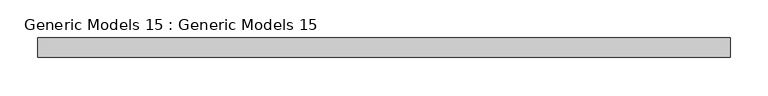
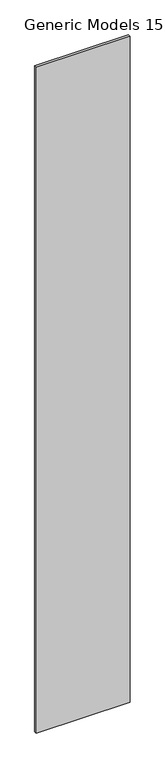
"""IFC4 building model written with IfcOpenShell, lengths in millimetres: proxy geometry, Generic Models 15 : Generic Models 15."""

from ifc_helpers import new_model, si_unit, frame, origin, place, context, project, spatial, polyline, outline, extrude, source, transform, mapped, element, save


def generic_models_15_generic_models_15_a6985b4b(model_context):
    return source(origin(), model_context, "Body", "SweptSolid", [
        extrude(outline(polyline([(-15207.3371373, -3405.661407), (-16121.7371373, -3405.661407), (-16121.7371373, -3380.261407), (-15207.3371373, -3380.261407), (-15207.3371373, -3405.661407)])), frame((0.0, 0.0, 304.8), z_axis=(0.0, 0.0, 1.0), x_axis=(1.0, 0.0, 0.0)), (0.0, 0.0, 1.0), 6858.0),
    ])


if __name__ == "__main__":
    model = new_model("IFC4")
    model_context = context("Model", 3, world=origin())
    ifc_project = project(units=[si_unit("LENGTHUNIT", "METRE", prefix="MILLI")], contexts=[model_context])
    site = spatial("IfcSite", under=ifc_project)
    building = spatial("IfcBuilding", under=site)
    placement = place(None, origin())
    generic_models_15_generic_models_15_shape = generic_models_15_generic_models_15_a6985b4b(model_context)
    element("IfcBuildingElementProxy", 1, Name="Generic Models 15 : Generic Models 15", ObjectType="Generic Models 15 : Generic Models 15", at=placement, inside=building, context=model_context, shape_type="MappedRepresentation", body=[
        mapped(generic_models_15_generic_models_15_shape, transform((0.0, 0.0, 0.0), x_axis=(1.0, 0.0, 0.0), y_axis=(0.0, 1.0, 0.0), z_axis=(0.0, 0.0, 1.0))),
    ])
    save(model, "model.ifc")

# Revit data of these elements
# Element 1 (IfcBuildingElementProxy, "Generic Models 15 : Generic Models 15")
#   Materials on its faces: "2.FRONT WALL PAINT"
# Materials
#   "2.FRONT WALL PAINT": class "Generic", colour RGB 120 120 120, transparency 0, Cost = 0
